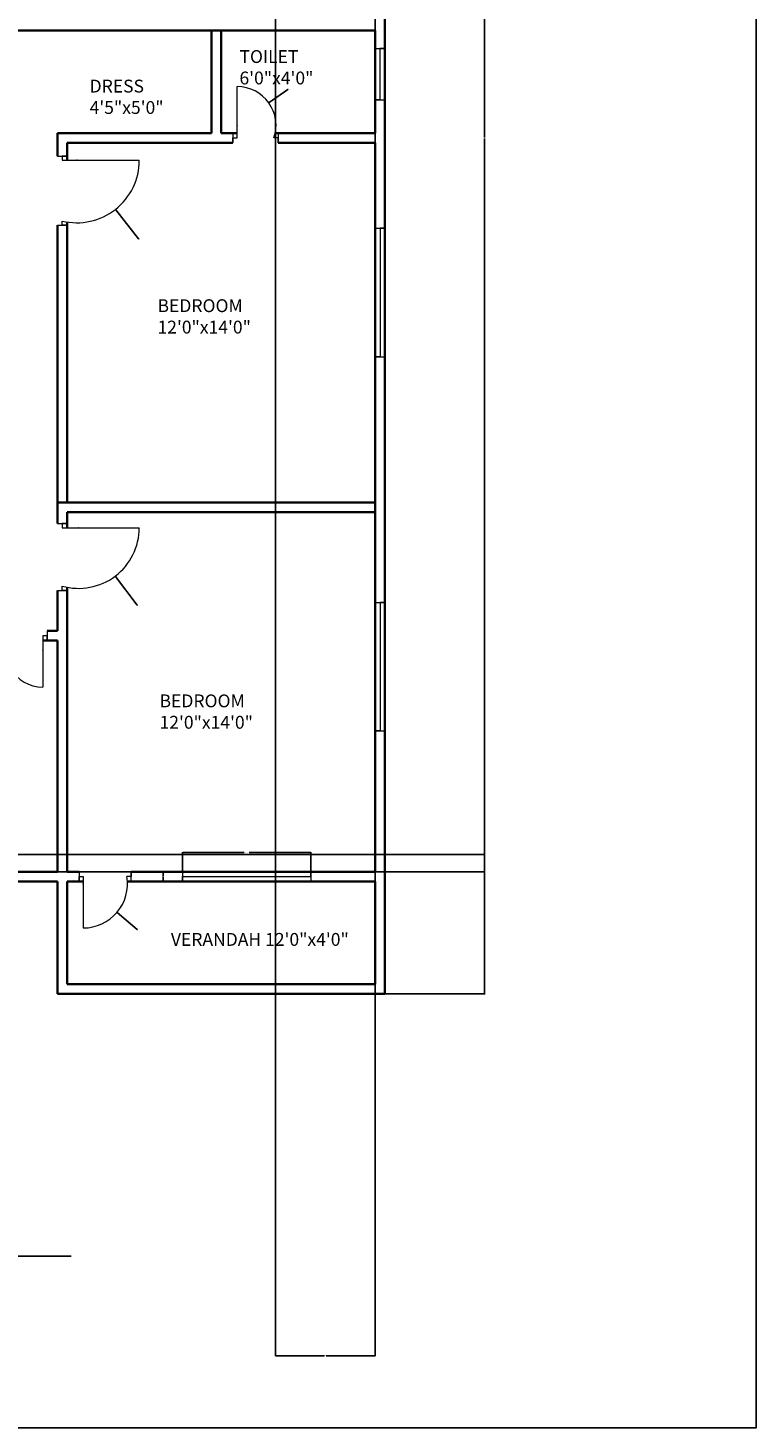
# Model space of a CAD drawing. Units: inches. Extents: x 1865 to 2795, y 1308 to 2437.
# Tile 2 of 3: x 2455 to 2795, y 1308 to 1962. Entities that reach past the tile are written whole.
import ezdxf

# ---------------------------------------------------------------- set-up
doc = ezdxf.new("R2010")
doc.units = ezdxf.units.IN
for name, color, linetype, lineweight in [('A-ANNO-DIMS', 2, 'Continuous', 18), ('A-ANNO-TTLB', 7, 'Continuous', 25), ('A-AREA-IDEN', 7, 'Continuous', 18), ('A-DOOR', 3, 'Continuous', 18), ('A-GLAZ', 4, 'Continuous', 18), ('A-WALL', 7, 'Continuous', 35)]:
    doc.layers.add(name, color=color, linetype=linetype, lineweight=lineweight)
doc.styles.get("Standard").update_dxf_attribs({"font": 'arial.ttf'})
doc.dimstyles.get("Standard").update_dxf_attribs({"dimtxt": 0.18, "dimasz": 0.18, "dimexe": 0.18, "dimexo": 0.0625, "dimgap": 0.09, "dimtad": 0, "dimtih": 1, "dimtoh": 1, "dimdec": 4, "dimzin": 0, "dimdsep": 46, "dimtxsty": 'Standard', "dimcen": 0.09, "dimadec": 0, "dimazin": 0, "dimtfac": 1, "dimtdec": 4, "dimtofl": 0, "dimtmove": 0, "dimatfit": 3, "dimfxl": 1, "dimtolj": 1, "dimtzin": 0, "dimarcsym": 0})

# ---------------------------------------------------------------- blocks, each defined once
blk = doc.blocks.new('WIN-60IN')
for p, q in [((0, 4.5), (0, 0)), ((0, 0), (0, 2.25)), ((0, 2.25), (60, 2.25)), ((60, 2.25), (60, 4.5)), ((60, 4.5), (60, 0))]:
    blk.add_line(p, q)
blk = doc.blocks.new('*D4')
at = {"layer": 'A-ANNO-DIMS', "color": 0, "lineweight": -2, "transparency": 16777216}
for p, q in [((2527.26, 1568.22), (2527.26, 1577.34)), ((2527.44, 1577.16), (2556.14, 1577.16)), ((2587.08, 1577.16), (2558.38, 1577.16)), ((2587.26, 1568.22), (2587.26, 1577.34))]:
    blk.add_line(p, q, dxfattribs=at)
at = {"layer": 'A-ANNO-DIMS', "color": 0, "transparency": 16777216}
for points in [[(2527.44, 1577.19), (2527.44, 1577.13), (2527.26, 1577.16)], [(2587.08, 1577.19), (2587.08, 1577.13), (2587.26, 1577.16)]]:
    blk.add_solid(points, dxfattribs=at)
at = {"layer": 'Defpoints', "color": 0, "transparency": 16777216}
for p in [(2587.26, 1577.16), (2527.26, 1568.16), (2587.26, 1568.16)]:
    blk.add_point(p, dxfattribs=at)
at = {"layer": 'A-ANNO-DIMS', "color": 0, "transparency": 16777216, "insert": (2557.26, 1577.16), "char_height": 0.18, "attachment_point": 5}
blk.add_mtext('\\A1;WINDOW 60 TYP.', dxfattribs=at)
blk = doc.blocks.new('*D5')
at = {"layer": 'A-ANNO-DIMS', "color": 0, "lineweight": -2, "transparency": 16777216}
for p, q in [((2527.2, 1568.16), (2518.08, 1568.16)), ((2527.2, 1563.66), (2518.08, 1563.66)), ((2518.26, 1567.98), (2518.26, 1566.09)), ((2518.26, 1563.84), (2518.26, 1565.72))]:
    blk.add_line(p, q, dxfattribs=at)
at = {"layer": 'A-ANNO-DIMS', "color": 0, "transparency": 16777216}
for points in [[(2518.23, 1567.98), (2518.29, 1567.98), (2518.26, 1568.16)], [(2518.23, 1563.84), (2518.29, 1563.84), (2518.26, 1563.66)]]:
    blk.add_solid(points, dxfattribs=at)
at = {"layer": 'Defpoints', "color": 0, "transparency": 16777216}
for p in [(2518.26, 1568.16), (2527.26, 1568.16), (2527.26, 1563.66)]:
    blk.add_point(p, dxfattribs=at)
at = {"layer": 'A-ANNO-DIMS', "color": 0, "transparency": 16777216, "insert": (2518.26, 1565.91), "char_height": 0.18, "attachment_point": 5}
blk.add_mtext('\\A1;5 TYP.', dxfattribs=at)
blk = doc.blocks.new('*D11')
at = {"layer": 'A-ANNO-DIMS', "color": 0, "lineweight": -2, "transparency": 16777216}
for p, q in [((2621.9, 2310.66), (2668.62, 2310.66)), ((2668.44, 2310.48), (2668.44, 1911.09)), ((2668.44, 1511.34), (2668.44, 1910.72)), ((2621.9, 1511.16), (2668.62, 1511.16))]:
    blk.add_line(p, q, dxfattribs=at)
at = {"layer": 'A-ANNO-DIMS', "color": 0, "transparency": 16777216}
for points in [[(2668.41, 2310.48), (2668.47, 2310.48), (2668.44, 2310.66)], [(2668.41, 1511.34), (2668.47, 1511.34), (2668.44, 1511.16)]]:
    blk.add_solid(points, dxfattribs=at)
at = {"layer": 'Defpoints', "color": 0, "transparency": 16777216}
for p in [(2621.84, 2310.66), (2668.44, 2310.66), (2621.84, 1511.16)]:
    blk.add_point(p, dxfattribs=at)
at = {"layer": 'A-ANNO-DIMS', "color": 0, "transparency": 16777216, "insert": (2668.44, 1910.91), "char_height": 0.18, "attachment_point": 5}
blk.add_mtext('\\A1;799.5', dxfattribs=at)
blk = doc.blocks.new('*D15')
at = {"layer": 'A-ANNO-DIMS', "color": 0, "lineweight": -2, "transparency": 16777216}
for p, q in [((2570.72, 2306.09), (2570.72, 1341.86)), ((2617.34, 2306.09), (2617.34, 1341.86)), ((2570.9, 1342.04), (2593.65, 1342.04)), ((2617.16, 1342.04), (2594.41, 1342.04))]:
    blk.add_line(p, q, dxfattribs=at)
at = {"layer": 'A-ANNO-DIMS', "color": 0, "transparency": 16777216}
for points in [[(2570.9, 1342.07), (2570.9, 1342.01), (2570.72, 1342.04)], [(2617.16, 1342.07), (2617.16, 1342.01), (2617.34, 1342.04)]]:
    blk.add_solid(points, dxfattribs=at)
at = {"layer": 'Defpoints', "color": 0, "transparency": 16777216}
for p in [(2570.72, 2306.16), (2617.34, 2306.16), (2617.34, 1342.04)]:
    blk.add_point(p, dxfattribs=at)
at = {"layer": 'A-ANNO-DIMS', "color": 0, "transparency": 16777216, "insert": (2594.03, 1342.04), "char_height": 0.18, "attachment_point": 5}
blk.add_mtext('\\A1;46.61', dxfattribs=at)
blk = doc.blocks.new('*D28')
at = {"layer": 'A-ANNO-DIMS', "color": 0, "lineweight": -2, "transparency": 16777216}
for p, q in [((2279.9, 1576.16), (2668.62, 1576.16)), ((2668.44, 1575.98), (2668.44, 1572.34)), ((2668.44, 1568.34), (2668.44, 1571.97)), ((2279.9, 1568.16), (2668.62, 1568.16))]:
    blk.add_line(p, q, dxfattribs=at)
at = {"layer": 'A-ANNO-DIMS', "color": 0, "transparency": 16777216}
for points in [[(2668.41, 1575.98), (2668.47, 1575.98), (2668.44, 1576.16)], [(2668.41, 1568.34), (2668.47, 1568.34), (2668.44, 1568.16)]]:
    blk.add_solid(points, dxfattribs=at)
at = {"layer": 'Defpoints', "color": 0, "transparency": 16777216}
for p in [(2279.84, 1576.16), (2668.44, 1576.16), (2279.84, 1568.16)]:
    blk.add_point(p, dxfattribs=at)
at = {"layer": 'A-ANNO-DIMS', "color": 0, "transparency": 16777216, "insert": (2668.44, 1572.16), "char_height": 0.18, "attachment_point": 5}
blk.add_mtext('\\A1;8', dxfattribs=at)
blk = doc.blocks.new('*D31')
at = {"layer": 'A-ANNO-DIMS', "color": 0, "lineweight": -2, "transparency": 16777216}
for p, q in [((2477.83, 1900.47), (2478.01, 1900.47)), ((2477.92, 1900.38), (2477.92, 1900.56)), ((2506.8, 1863.81), (2496.08, 1877.42)), ((2506.98, 1863.81), (2506.8, 1863.81))]:
    blk.add_line(p, q, dxfattribs=at)
at = {"layer": 'A-ANNO-DIMS', "color": 0, "transparency": 16777216}
blk.add_solid([(2496.1, 1877.43), (2496.06, 1877.4), (2495.97, 1877.56)], dxfattribs=at)
at = {"layer": 'Defpoints', "color": 0, "transparency": 16777216}
for p in [(2477.92, 1900.47), (2495.97, 1877.56)]:
    blk.add_point(p, dxfattribs=at)
at = {"layer": 'A-ANNO-DIMS', "color": 0, "transparency": 16777216, "insert": (2507.46, 1863.81), "char_height": 0.18, "attachment_point": 5}
blk.add_mtext('\\A1;R29.17', dxfattribs=at)
blk = doc.blocks.new('*D35')
at = {"layer": 'A-ANNO-DIMS', "color": 0, "lineweight": -2, "transparency": 16777216}
for p, q in [((2478.7, 1728.83), (2478.88, 1728.83)), ((2478.79, 1728.74), (2478.79, 1728.92)), ((2506.11, 1692.72), (2495.97, 1706.11)), ((2506.29, 1692.72), (2506.11, 1692.72))]:
    blk.add_line(p, q, dxfattribs=at)
at = {"layer": 'A-ANNO-DIMS', "color": 0, "transparency": 16777216}
blk.add_solid([(2495.99, 1706.13), (2495.95, 1706.1), (2495.86, 1706.26)], dxfattribs=at)
at = {"layer": 'Defpoints', "color": 0, "transparency": 16777216}
for p in [(2478.79, 1728.83), (2495.86, 1706.26)]:
    blk.add_point(p, dxfattribs=at)
at = {"layer": 'A-ANNO-DIMS', "color": 0, "transparency": 16777216, "insert": (2506.7, 1692.72), "char_height": 0.18, "attachment_point": 5}
blk.add_mtext('\\A1;R28.3', dxfattribs=at)
blk = doc.blocks.new('*D43')
at = {"layer": 'A-ANNO-DIMS', "color": 0, "lineweight": -2, "transparency": 16777216}
for p, q in [((2480.85, 1562.52), (2481.03, 1562.52)), ((2480.94, 1562.43), (2480.94, 1562.61)), ((2506.11, 1541.2), (2496.81, 1549.08)), ((2506.29, 1541.2), (2506.11, 1541.2))]:
    blk.add_line(p, q, dxfattribs=at)
at = {"layer": 'A-ANNO-DIMS', "color": 0, "transparency": 16777216}
blk.add_solid([(2496.83, 1549.1), (2496.79, 1549.06), (2496.67, 1549.2)], dxfattribs=at)
at = {"layer": 'Defpoints', "color": 0, "transparency": 16777216}
for p in [(2480.94, 1562.52), (2496.67, 1549.2)]:
    blk.add_point(p, dxfattribs=at)
at = {"layer": 'A-ANNO-DIMS', "color": 0, "transparency": 16777216, "insert": (2506.84, 1541.2), "char_height": 0.18, "attachment_point": 5}
blk.add_mtext('\\A1;R20.615', dxfattribs=at)
blk = doc.blocks.new('*D48')
at = {"layer": 'A-ANNO-DIMS', "color": 0, "lineweight": -2, "transparency": 16777216}
for p, q in [((2576.46, 1933.62), (2567.76, 1927.42)), ((2576.64, 1933.62), (2576.46, 1933.62)), ((2552.79, 1916.8), (2552.97, 1916.8)), ((2552.88, 1916.71), (2552.88, 1916.89))]:
    blk.add_line(p, q, dxfattribs=at)
at = {"layer": 'A-ANNO-DIMS', "color": 0, "transparency": 16777216}
blk.add_solid([(2567.74, 1927.44), (2567.78, 1927.39), (2567.62, 1927.31)], dxfattribs=at)
at = {"layer": 'Defpoints', "color": 0, "transparency": 16777216}
for p in [(2567.62, 1927.31), (2552.88, 1916.8)]:
    blk.add_point(p, dxfattribs=at)
at = {"layer": 'A-ANNO-DIMS', "color": 0, "transparency": 16777216, "insert": (2577.19, 1933.62), "char_height": 0.18, "attachment_point": 5}
blk.add_mtext('\\A1;R18.106', dxfattribs=at)
blk = doc.blocks.new('*D49')
at = {"layer": 'A-ANNO-DIMS', "color": 0, "lineweight": -2, "transparency": 16777216}
for p, q in [((2461.87, 1671.78), (2462.05, 1671.78)), ((2461.96, 1671.69), (2461.96, 1671.87)), ((2437.81, 1658.01), (2446.71, 1663.08)), ((2437.63, 1658.01), (2437.81, 1658.01))]:
    blk.add_line(p, q, dxfattribs=at)
at = {"layer": 'A-ANNO-DIMS', "color": 0, "transparency": 16777216}
blk.add_solid([(2446.7, 1663.11), (2446.73, 1663.06), (2446.87, 1663.17)], dxfattribs=at)
at = {"layer": 'Defpoints', "color": 0, "transparency": 16777216}
for p in [(2461.96, 1671.78), (2446.87, 1663.17)]:
    blk.add_point(p, dxfattribs=at)
at = {"layer": 'A-ANNO-DIMS', "color": 0, "transparency": 16777216, "insert": (2437.09, 1658.01), "char_height": 0.18, "attachment_point": 5}
blk.add_mtext('\\A1;R17.372', dxfattribs=at)

msp = doc.modelspace()

# ---------------------------------------------------------------- linework, layer by layer
at = {"layer": 'A-ANNO-TTLB'}
msp.add_line((2132.0289, 1388.6384), (2475.3371, 1388.6384), dxfattribs=at)
msp.add_lwpolyline([(1865.3404, 2436.9121), (2795.2369, 2436.9121), (2795.2369, 1308.3367), (1865.3404, 1308.3367)], close=True, dxfattribs=at)
at = {"layer": 'A-DOOR'}
for p, q in [((2552.8757, 1910.9064), (2552.8757, 1934.9064)), ((2550.8757, 1913.1564), (2550.8757, 1908.6564)), ((2550.8757, 1908.6564), (2550.8757, 1910.9064)), ((2550.8757, 1910.9064), (2552.8757, 1910.9064)), ((2571.995, 1910.9064), (2569.995, 1910.9064)), ((2571.995, 1913.1564), (2571.995, 1908.6564)), ((2571.995, 1908.6564), (2571.995, 1910.9064)), ((2468.8379, 1902.4715), (2473.3379, 1902.4715)), ((2473.3379, 1902.4715), (2471.0879, 1902.4715)), ((2471.0879, 1902.4715), (2471.0879, 1900.4715)), ((2471.0879, 1900.4715), (2507.0879, 1900.4715)), ((2471.0879, 1870.1112), (2471.0879, 1872.1112)), ((2468.8379, 1870.1112), (2473.3379, 1870.1112)), ((2473.3379, 1870.1112), (2471.0879, 1870.1112)), ((2468.8379, 1730.8282), (2473.3379, 1730.8282)), ((2473.3379, 1730.8282), (2471.0879, 1730.8282)), ((2471.0879, 1730.8282), (2471.0879, 1728.8282)), ((2471.0879, 1728.8282), (2507.0879, 1728.8282)), ((2471.0879, 1699.595), (2471.0879, 1701.595)), ((2468.8379, 1699.595), (2473.3379, 1699.595)), ((2473.3379, 1699.595), (2471.0879, 1699.595)), ((2463.9959, 1680.6564), (2463.9959, 1676.1564)), ((2463.9959, 1678.4064), (2461.9959, 1678.4064)), ((2461.9959, 1678.4064), (2461.9959, 1654.4064)), ((2463.9959, 1676.1564), (2463.9959, 1678.4064)), ((2478.9415, 1568.1564), (2478.9415, 1563.6564)), ((2478.9415, 1563.6564), (2478.9415, 1565.9064)), ((2478.9415, 1565.9064), (2480.9415, 1565.9064)), ((2480.9415, 1565.9064), (2480.9415, 1541.9064)), ((2503.2762, 1565.9064), (2501.2762, 1565.9064)), ((2503.2762, 1563.6564), (2503.2762, 1568.1564)), ((2503.2762, 1568.1564), (2503.2762, 1565.9064))]:
    msp.add_line(p, q, dxfattribs=at)
for centre, radius, start, end in [((2552.8757, 1916.8008), 18.1057, 341.0009784, 90), ((2477.9169, 1900.4715), 29.171, 256.4611761, 0), ((2478.7872, 1728.8282), 28.3007, 254.2134267, 0), ((2461.9604, 1671.7785), 17.3721, 149.2662645, 270.1168983), ((2480.9415, 1562.521), 20.6145, 270, 9.4523176)]:
    msp.add_arc(centre, radius, start, end, dxfattribs=at)
at = {"layer": 'A-GLAZ'}
for p, q in [((2617.3379, 1952.6552), (2619.9827, 1952.6552)), ((2621.8379, 1952.6552), (2619.5218, 1952.6552)), ((2619.5218, 1952.6552), (2619.5218, 1928.6552)), ((2619.9827, 1952.6552), (2621.8379, 1952.6552)), ((2619.5218, 1928.6552), (2617.3379, 1928.6552)), ((2617.3379, 1928.6552), (2621.8379, 1928.6552))]:
    msp.add_line(p, q, dxfattribs=at)
at = {"layer": 'A-WALL'}
for p, q in [((2621.8379, 2310.6564), (2621.8379, 1511.1564)), ((2363.0176, 1961.1564), (2473.3379, 1961.1564)), ((2473.3379, 1961.1564), (2617.3379, 1961.1564)), ((2540.8379, 1961.1564), (2540.8379, 1913.1564)), ((2545.3379, 1961.1564), (2545.3379, 1913.1564)), ((2617.3379, 1961.1564), (2617.3379, 1913.1564)), ((2468.8379, 1913.1564), (2540.8379, 1913.1564)), ((2468.8379, 1913.1564), (2468.8379, 1902.4715)), ((2545.3379, 1913.1564), (2552.8757, 1913.1564)), ((2570.6108, 1913.1564), (2617.3379, 1913.1564)), ((2473.3379, 1908.6564), (2550.8757, 1908.6564)), ((2473.3379, 1908.6564), (2473.3379, 1900.4715)), ((2571.995, 1908.6564), (2617.3379, 1908.6564)), ((2617.3379, 1908.6564), (2617.3379, 1568.1564)), ((2473.3379, 1871.6622), (2473.3379, 1740.6564)), ((2468.8379, 1870.1112), (2468.8379, 1730.8282)), ((2468.8379, 1740.6564), (2473.3379, 1740.6564)), ((2473.3379, 1740.6564), (2617.3379, 1740.6564)), ((2473.3379, 1736.1564), (2617.3379, 1736.1564)), ((2473.3379, 1736.1564), (2473.3379, 1728.8282)), ((2473.3379, 1701.0571), (2473.3379, 1568.1564)), ((2468.8379, 1699.595), (2468.8379, 1680.6564)), ((2468.8379, 1680.6564), (2463.9959, 1680.6564)), ((2461.9959, 1676.1564), (2468.8379, 1676.1564)), ((2468.8379, 1676.1564), (2468.8379, 1568.1564)), ((2468.8379, 1568.1564), (2384.8379, 1568.1564)), ((2384.8379, 1568.1564), (2468.8379, 1568.1564)), ((2384.8379, 1563.6564), (2468.8379, 1563.6564)), ((2468.8379, 1563.6564), (2468.8379, 1511.1564)), ((2473.3379, 1568.1564), (2478.9415, 1568.1564)), ((2473.3379, 1563.6564), (2480.9415, 1563.6564)), ((2473.3379, 1563.6564), (2473.3379, 1515.6564)), ((2501.5247, 1563.6564), (2617.3379, 1563.6564)), ((2503.2762, 1568.1564), (2617.3379, 1568.1564)), ((2617.3379, 1563.6564), (2617.3379, 1515.6564)), ((2468.8379, 1511.1564), (2617.3379, 1511.1564)), ((2473.3379, 1515.6564), (2617.3379, 1515.6564)), ((2473.3379, 1515.6564), (2617.3379, 1515.6564)), ((2473.3379, 1511.1564), (2621.8379, 1511.1564))]:
    msp.add_line(p, q, dxfattribs=at)

# ---------------------------------------------------------------- block references
at = {"layer": 'A-GLAZ', "extrusion": (0, 0, -1), "zscale": -1, "rotation": 270}
for p in [(-2621.8383, 1868.7455), (-2621.8383, 1693.9407)]:
    msp.add_blockref('WIN-60IN', p, dxfattribs=at)
at = {"layer": 'A-GLAZ'}
msp.add_blockref('WIN-60IN', (2527.26, 1563.656), dxfattribs=at)

# ---------------------------------------------------------------- texts
at = {"layer": 'A-AREA-IDEN', "char_height": 6, "attachment_point": 1}
for s, width, insert in [('TOILET\\P6\'0"x4\'0"', 114.756698, (2553.9009, 1951.9372)), ('DRESS\\P4\'5"x5\'0"', 133.455893, (2483.882, 1938.143)), ('BEDROOM\\P12\'0"x14\'0"', 154.985598, (2515.6063, 1835.5688)), ('BEDROOM\\P12\'0"x14\'0"', 154.985598, (2516.5577, 1650.9809)), ('VERANDAH 12\'0"x4\'0"', 172.928349, (2521.861, 1539.5578))]:
    msp.add_mtext_dynamic_manual_height_columns(s, width=width, gutter_width=12.5, heights=[0], dxfattribs=dict(at, insert=insert))

# ---------------------------------------------------------------- dimensions: what is measured, and where the dimension line sits
at = {"layer": 'A-ANNO-DIMS'}
for base, p1, p2, override, picture, middle in [((2668.4379, 2310.6564), (2621.8379, 1511.1564), (2621.8379, 2310.6564), {"dimdec": 1, "dimlfac": 1, "dimrnd": 0, "dimzin": 0, "dimdsep": 46, "dimlunit": 2}, '*D11', (2668.4379, 1910.9064)), ((2668.4379, 1576.1564), (2279.8379, 1568.1564), (2279.8379, 1576.1564), {"dimdec": 0, "dimlfac": 1, "dimrnd": 0, "dimzin": 0, "dimdsep": 46, "dimlunit": 2}, '*D28', (2668.4379, 1572.1564))]:
    dim = msp.add_linear_dim(base=base, p1=p1, p2=p2, angle=90, dimstyle='Standard', override=override, dxfattribs=at)
    dim.commit()
    dim.dimension.update_dxf_attribs({"geometry": picture, "text_midpoint": middle})
dim = msp.add_linear_dim(base=(2617.3379, 1342.0384), p1=(2570.7247, 2306.1564), p2=(2617.3379, 2306.1564), dimstyle='Standard', override={"dimdec": 2, "dimlfac": 1, "dimrnd": 0, "dimzin": 0, "dimdsep": 46, "dimlunit": 2}, dxfattribs=at)
dim.commit()
dim.dimension.update_dxf_attribs({"geometry": '*D15', "text_midpoint": (2594.0313, 1342.0384)})
for center, mpoint, override, picture, middle in [((2552.8757, 1916.8008), (2567.6158, 1927.3148), {"dimdec": 3, "dimlfac": 1, "dimrnd": 0, "dimzin": 0, "dimdsep": 46, "dimlunit": 2}, '*D48', (2577.1895, 1933.6233)), ((2477.9169, 1900.4715), (2495.9689, 1877.5571), {"dimdec": 2, "dimlfac": 1, "dimrnd": 0, "dimzin": 0, "dimdsep": 46, "dimlunit": 2}, '*D31', (2507.46, 1863.8085)), ((2478.7872, 1728.8282), (2495.861, 1706.258), {"dimdec": 1, "dimlfac": 1, "dimrnd": 0, "dimzin": 0, "dimdsep": 46, "dimlunit": 2}, '*D35', (2506.6952, 1692.7159)), ((2461.9604, 1671.7785), (2446.869, 1663.174), {"dimdec": 3, "dimlfac": 1, "dimrnd": 0, "dimzin": 0, "dimdsep": 46, "dimlunit": 2}, '*D49', (2437.0853, 1658.0113)), ((2480.9415, 1562.521), (2496.6699, 1549.1951), {"dimdec": 3, "dimlfac": 1, "dimrnd": 0, "dimzin": 0, "dimdsep": 46, "dimlunit": 2}, '*D43', (2506.8373, 1541.1996))]:
    dim = msp.add_radius_dim(center=center, mpoint=mpoint, dimstyle='Standard', override=override, dxfattribs=at)
    dim.commit()
    dim.dimension.update_dxf_attribs({"geometry": picture, "text_midpoint": middle, "dimtype": 164})
dim = msp.add_linear_dim(base=(2587.2598, 1577.1564), p1=(2527.2598, 1568.1564), p2=(2587.2598, 1568.1564), text='WINDOW <> TYP.', dimstyle='Standard', override={"dimdec": 0, "dimlfac": 1, "dimrnd": 0, "dimzin": 0, "dimdsep": 46, "dimlunit": 2}, dxfattribs=at)
dim.commit()
dim.dimension.update_dxf_attribs({"geometry": '*D4', "text_midpoint": (2557.2598, 1577.1564)})
dim = msp.add_linear_dim(base=(2518.2597871184, 1568.1564380793), p1=(2527.2597871184, 1563.6564380793), p2=(2527.2597871184, 1568.1564380793), angle=90, text='<> TYP.', dimstyle='Standard', override={"dimdec": 0, "dimlfac": 1, "dimrnd": 0, "dimzin": 0, "dimdsep": 46, "dimlunit": 2}, dxfattribs=at)
dim.commit()
dim.dimension.update_dxf_attribs({"geometry": '*D5', "text_midpoint": (2518.2597871184, 1565.9064380793)})

doc.saveas('drawing.dxf')
